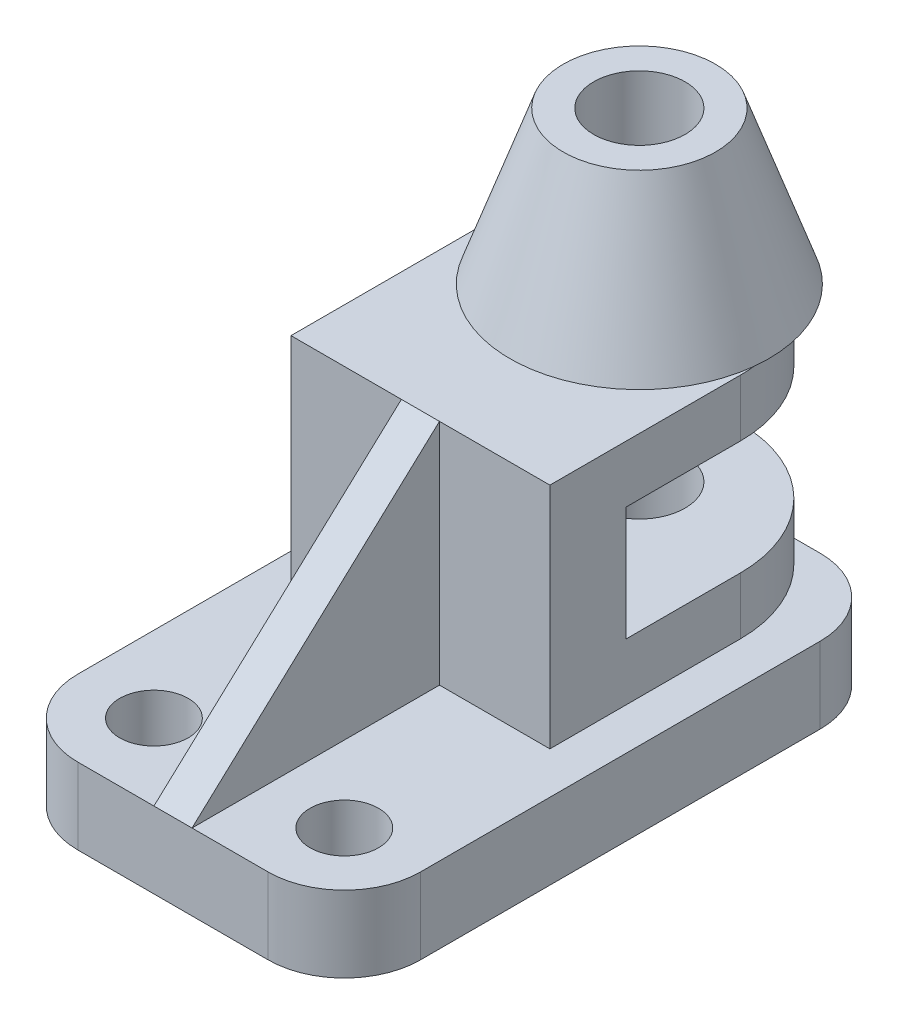
ISO-10303-21;
HEADER;
FILE_DESCRIPTION(('STEP AP214'),'2;1');
FILE_NAME('part.step','',(''),(''),'','','');
FILE_SCHEMA(('AUTOMOTIVE_DESIGN { 1 0 10303 214 1 1 1 1 }'));
ENDSEC;
DATA;
#1=APPLICATION_CONTEXT('core data for automotive mechanical design processes');
#2=APPLICATION_PROTOCOL_DEFINITION('international standard','automotive_design',2000,#1);
#3=PRODUCT_CONTEXT('',#1,'mechanical');
#4=PRODUCT('Part','Part','',(#3));
#5=PRODUCT_RELATED_PRODUCT_CATEGORY('part','',(#4));
#6=PRODUCT_DEFINITION_FORMATION('','',#4);
#7=PRODUCT_DEFINITION_CONTEXT('part definition',#1,'design');
#8=PRODUCT_DEFINITION('design','',#6,#7);
#9=PRODUCT_DEFINITION_SHAPE('','',#8);
#10=(LENGTH_UNIT() NAMED_UNIT(*) SI_UNIT(.MILLI.,.METRE.));
#11=(NAMED_UNIT(*) PLANE_ANGLE_UNIT() SI_UNIT($,.RADIAN.));
#12=(NAMED_UNIT(*) SI_UNIT($,.STERADIAN.) SOLID_ANGLE_UNIT());
#13=UNCERTAINTY_MEASURE_WITH_UNIT(LENGTH_MEASURE(1.E-05),#10,'distance_accuracy_value','');
#14=(GEOMETRIC_REPRESENTATION_CONTEXT(3) GLOBAL_UNCERTAINTY_ASSIGNED_CONTEXT((#13)) GLOBAL_UNIT_ASSIGNED_CONTEXT((#10,
#11,#12)) REPRESENTATION_CONTEXT('',''));
#15=CARTESIAN_POINT('',(0.,0.,0.));
#16=DIRECTION('',(0.,0.,1.));
#17=DIRECTION('',(1.,0.,0.));
#18=AXIS2_PLACEMENT_3D('',#15,#16,#17);
#19=CARTESIAN_POINT('',(0.,20.,0.));
#20=DIRECTION('',(0.,-1.,0.));
#21=DIRECTION('',(0.,0.,-1.));
#22=AXIS2_PLACEMENT_3D('',#19,#20,#21);
#23=PLANE('',#22);
#24=CARTESIAN_POINT('',(-25.,20.,52.5));
#25=DIRECTION('',(0.,1.,0.));
#26=DIRECTION('',(0.,0.,1.));
#27=AXIS2_PLACEMENT_3D('',#24,#25,#26);
#28=CIRCLE('',#27,9.);
#29=CARTESIAN_POINT('',(-25.,20.,61.5));
#30=VERTEX_POINT('',#29);
#31=EDGE_CURVE('E240',#30,#30,#28,.T.);
#32=ORIENTED_EDGE('',*,*,#31,.F.);
#33=EDGE_LOOP('',(#32));
#34=FACE_BOUND('',#33,.T.);
#35=DIRECTION('',(0.,0.,1.));
#36=VECTOR('',#35,1.);
#37=CARTESIAN_POINT('',(-5.,20.,0.));
#38=LINE('',#37,#36);
#39=CARTESIAN_POINT('',(-5.,20.,7.50000000000001));
#40=VERTEX_POINT('',#39);
#41=CARTESIAN_POINT('',(-5.,20.,72.5));
#42=VERTEX_POINT('',#41);
#43=EDGE_CURVE('E186',#40,#42,#38,.T.);
#44=ORIENTED_EDGE('',*,*,#43,.F.);
#45=DIRECTION('',(1.,0.,0.));
#46=VECTOR('',#45,1.);
#47=CARTESIAN_POINT('',(-34.,20.,7.50000000000001));
#48=LINE('',#47,#46);
#49=CARTESIAN_POINT('',(-34.,20.,7.50000000000001));
#50=VERTEX_POINT('',#49);
#51=EDGE_CURVE('E507',#50,#40,#48,.T.);
#52=ORIENTED_EDGE('',*,*,#51,.F.);
#53=DIRECTION('',(0.,0.,1.));
#54=VECTOR('',#53,1.);
#55=CARTESIAN_POINT('',(-34.,20.,-42.5));
#56=LINE('',#55,#54);
#57=CARTESIAN_POINT('',(-34.,20.,-42.5));
#58=VERTEX_POINT('',#57);
#59=EDGE_CURVE('E492',#58,#50,#56,.T.);
#60=ORIENTED_EDGE('',*,*,#59,.F.);
#61=CARTESIAN_POINT('',(0.,20.,-42.5));
#62=DIRECTION('',(0.,1.,0.));
#63=DIRECTION('',(0.,0.,1.));
#64=AXIS2_PLACEMENT_3D('',#61,#62,#63);
#65=CIRCLE('',#64,34.);
#66=CARTESIAN_POINT('',(-16.,20.,-72.5));
#67=VERTEX_POINT('',#66);
#68=EDGE_CURVE('E11',#67,#58,#65,.T.);
#69=ORIENTED_EDGE('',*,*,#68,.F.);
#70=DIRECTION('',(-1.,0.,0.));
#71=VECTOR('',#70,1.);
#72=CARTESIAN_POINT('',(-45.,20.,-72.5));
#73=LINE('',#72,#71);
#74=CARTESIAN_POINT('',(-25.,20.,-72.5));
#75=VERTEX_POINT('',#74);
#76=EDGE_CURVE('E225',#67,#75,#73,.T.);
#77=ORIENTED_EDGE('',*,*,#76,.T.);
#78=CARTESIAN_POINT('',(-25.,20.,-52.5));
#79=DIRECTION('',(0.,-1.,0.));
#80=DIRECTION('',(0.,0.,-1.));
#81=AXIS2_PLACEMENT_3D('',#78,#79,#80);
#82=CIRCLE('',#81,20.);
#83=CARTESIAN_POINT('',(-45.,20.,-52.5));
#84=VERTEX_POINT('',#83);
#85=EDGE_CURVE('E267',#75,#84,#82,.F.);
#86=ORIENTED_EDGE('',*,*,#85,.T.);
#87=DIRECTION('',(0.,0.,1.));
#88=VECTOR('',#87,1.);
#89=CARTESIAN_POINT('',(-45.,20.,72.5));
#90=LINE('',#89,#88);
#91=CARTESIAN_POINT('',(-45.,20.,52.5));
#92=VERTEX_POINT('',#91);
#93=EDGE_CURVE('E221',#84,#92,#90,.T.);
#94=ORIENTED_EDGE('',*,*,#93,.T.);
#95=CARTESIAN_POINT('',(-25.,20.,52.5));
#96=DIRECTION('',(0.,-1.,0.));
#97=DIRECTION('',(0.,0.,-1.));
#98=AXIS2_PLACEMENT_3D('',#95,#96,#97);
#99=CIRCLE('',#98,20.);
#100=CARTESIAN_POINT('',(-25.,20.,72.5));
#101=VERTEX_POINT('',#100);
#102=EDGE_CURVE('E217',#92,#101,#99,.F.);
#103=ORIENTED_EDGE('',*,*,#102,.T.);
#104=DIRECTION('',(1.,0.,0.));
#105=VECTOR('',#104,1.);
#106=CARTESIAN_POINT('',(-45.,20.,72.5));
#107=LINE('',#106,#105);
#108=EDGE_CURVE('E209',#101,#42,#107,.T.);
#109=ORIENTED_EDGE('',*,*,#108,.T.);
#110=EDGE_LOOP('',(#44,#52,#60,#69,#77,#86,#94,#103,#109));
#111=FACE_BOUND('',#110,.T.);
#112=ADVANCED_FACE('F43',(#34,#111),#23,.F.);
#113=CARTESIAN_POINT('',(-34.,80.,7.50000000000001));
#114=DIRECTION('',(0.,0.,-1.));
#115=DIRECTION('',(-1.,0.,0.));
#116=AXIS2_PLACEMENT_3D('',#113,#114,#115);
#117=PLANE('',#116);
#118=DIRECTION('',(0.,-1.,0.));
#119=VECTOR('',#118,1.);
#120=CARTESIAN_POINT('',(-5.,80.,7.50000000000001));
#121=LINE('',#120,#119);
#122=CARTESIAN_POINT('',(-5.,80.,7.49999999999999));
#123=VERTEX_POINT('',#122);
#124=EDGE_CURVE('E191',#123,#40,#121,.T.);
#125=ORIENTED_EDGE('',*,*,#124,.F.);
#126=DIRECTION('',(1.,0.,0.));
#127=VECTOR('',#126,1.);
#128=CARTESIAN_POINT('',(-34.,80.,7.50000000000001));
#129=LINE('',#128,#127);
#130=CARTESIAN_POINT('',(-34.,80.,7.50000000000001));
#131=VERTEX_POINT('',#130);
#132=EDGE_CURVE('E443',#131,#123,#129,.T.);
#133=ORIENTED_EDGE('',*,*,#132,.F.);
#134=DIRECTION('',(0.,-1.,0.));
#135=VECTOR('',#134,1.);
#136=CARTESIAN_POINT('',(-34.,80.,7.50000000000001));
#137=LINE('',#136,#135);
#138=EDGE_CURVE('E362',#131,#50,#137,.T.);
#139=ORIENTED_EDGE('',*,*,#138,.T.);
#140=ORIENTED_EDGE('',*,*,#51,.T.);
#141=EDGE_LOOP('',(#125,#133,#139,#140));
#142=FACE_BOUND('',#141,.T.);
#143=ADVANCED_FACE('F327',(#142),#117,.F.);
#144=CARTESIAN_POINT('',(-34.,80.,-42.5));
#145=DIRECTION('',(1.,0.,0.));
#146=DIRECTION('',(0.,0.,-1.));
#147=AXIS2_PLACEMENT_3D('',#144,#145,#146);
#148=PLANE('',#147);
#149=DIRECTION('',(0.,0.,1.));
#150=VECTOR('',#149,1.);
#151=CARTESIAN_POINT('',(-34.,35.,0.));
#152=LINE('',#151,#150);
#153=CARTESIAN_POINT('',(-34.,35.,-42.5));
#154=VERTEX_POINT('',#153);
#155=CARTESIAN_POINT('',(-34.,35.,-12.5));
#156=VERTEX_POINT('',#155);
#157=EDGE_CURVE('E473',#154,#156,#152,.T.);
#158=ORIENTED_EDGE('',*,*,#157,.F.);
#159=DIRECTION('',(0.,-1.,0.));
#160=VECTOR('',#159,1.);
#161=CARTESIAN_POINT('',(-34.,80.,-42.5));
#162=LINE('',#161,#160);
#163=EDGE_CURVE('E504',#154,#58,#162,.T.);
#164=ORIENTED_EDGE('',*,*,#163,.T.);
#165=ORIENTED_EDGE('',*,*,#59,.T.);
#166=ORIENTED_EDGE('',*,*,#138,.F.);
#167=DIRECTION('',(0.,0.,1.));
#168=VECTOR('',#167,1.);
#169=CARTESIAN_POINT('',(-34.,80.,-42.5));
#170=LINE('',#169,#168);
#171=CARTESIAN_POINT('',(-34.,80.,-42.5));
#172=VERTEX_POINT('',#171);
#173=EDGE_CURVE('E447',#172,#131,#170,.T.);
#174=ORIENTED_EDGE('',*,*,#173,.F.);
#175=CARTESIAN_POINT('',(-34.,65.,-42.5));
#176=VERTEX_POINT('',#175);
#177=EDGE_CURVE('E515',#172,#176,#162,.T.);
#178=ORIENTED_EDGE('',*,*,#177,.T.);
#179=DIRECTION('',(0.,0.,1.));
#180=VECTOR('',#179,1.);
#181=CARTESIAN_POINT('',(-34.,65.,0.));
#182=LINE('',#181,#180);
#183=CARTESIAN_POINT('',(-34.,65.,-12.5));
#184=VERTEX_POINT('',#183);
#185=EDGE_CURVE('E468',#176,#184,#182,.T.);
#186=ORIENTED_EDGE('',*,*,#185,.T.);
#187=DIRECTION('',(0.,1.,0.));
#188=VECTOR('',#187,1.);
#189=CARTESIAN_POINT('',(-34.,35.,-12.5));
#190=LINE('',#189,#188);
#191=EDGE_CURVE('E481',#156,#184,#190,.T.);
#192=ORIENTED_EDGE('',*,*,#191,.F.);
#193=EDGE_LOOP('',(#158,#164,#165,#166,#174,#178,#186,#192));
#194=FACE_BOUND('',#193,.T.);
#195=ADVANCED_FACE('F331',(#194),#148,.F.);
#196=CARTESIAN_POINT('',(34.,80.,7.50000000000001));
#197=DIRECTION('',(-1.,0.,0.));
#198=DIRECTION('',(0.,0.,1.));
#199=AXIS2_PLACEMENT_3D('',#196,#197,#198);
#200=PLANE('',#199);
#201=DIRECTION('',(0.,0.,-1.));
#202=VECTOR('',#201,1.);
#203=CARTESIAN_POINT('',(34.,35.,0.));
#204=LINE('',#203,#202);
#205=CARTESIAN_POINT('',(34.,35.,-12.5));
#206=VERTEX_POINT('',#205);
#207=CARTESIAN_POINT('',(34.,35.,-42.5));
#208=VERTEX_POINT('',#207);
#209=EDGE_CURVE('E480',#206,#208,#204,.T.);
#210=ORIENTED_EDGE('',*,*,#209,.F.);
#211=DIRECTION('',(0.,1.,0.));
#212=VECTOR('',#211,1.);
#213=CARTESIAN_POINT('',(34.,35.,-12.5));
#214=LINE('',#213,#212);
#215=CARTESIAN_POINT('',(34.,65.,-12.5));
#216=VERTEX_POINT('',#215);
#217=EDGE_CURVE('E489',#206,#216,#214,.T.);
#218=ORIENTED_EDGE('',*,*,#217,.T.);
#219=DIRECTION('',(0.,0.,-1.));
#220=VECTOR('',#219,1.);
#221=CARTESIAN_POINT('',(34.,65.,0.));
#222=LINE('',#221,#220);
#223=CARTESIAN_POINT('',(34.,65.,-42.5));
#224=VERTEX_POINT('',#223);
#225=EDGE_CURVE('E486',#216,#224,#222,.T.);
#226=ORIENTED_EDGE('',*,*,#225,.T.);
#227=DIRECTION('',(0.,-1.,0.));
#228=VECTOR('',#227,1.);
#229=CARTESIAN_POINT('',(34.,80.,-42.5));
#230=LINE('',#229,#228);
#231=CARTESIAN_POINT('',(34.,80.,-42.5));
#232=VERTEX_POINT('',#231);
#233=EDGE_CURVE('E517',#232,#224,#230,.T.);
#234=ORIENTED_EDGE('',*,*,#233,.F.);
#235=DIRECTION('',(0.,0.,-1.));
#236=VECTOR('',#235,1.);
#237=CARTESIAN_POINT('',(34.,80.,7.50000000000001));
#238=LINE('',#237,#236);
#239=CARTESIAN_POINT('',(34.,80.,7.50000000000001));
#240=VERTEX_POINT('',#239);
#241=EDGE_CURVE('E497',#240,#232,#238,.T.);
#242=ORIENTED_EDGE('',*,*,#241,.F.);
#243=DIRECTION('',(0.,-1.,0.));
#244=VECTOR('',#243,1.);
#245=CARTESIAN_POINT('',(34.,80.,7.50000000000001));
#246=LINE('',#245,#244);
#247=CARTESIAN_POINT('',(34.,20.,7.50000000000001));
#248=VERTEX_POINT('',#247);
#249=EDGE_CURVE('E444',#240,#248,#246,.T.);
#250=ORIENTED_EDGE('',*,*,#249,.T.);
#251=DIRECTION('',(0.,0.,-1.));
#252=VECTOR('',#251,1.);
#253=CARTESIAN_POINT('',(34.,20.,7.50000000000001));
#254=LINE('',#253,#252);
#255=CARTESIAN_POINT('',(34.,20.,-42.5));
#256=VERTEX_POINT('',#255);
#257=EDGE_CURVE('E510',#248,#256,#254,.T.);
#258=ORIENTED_EDGE('',*,*,#257,.T.);
#259=EDGE_CURVE('E513',#208,#256,#230,.T.);
#260=ORIENTED_EDGE('',*,*,#259,.F.);
#261=EDGE_LOOP('',(#210,#218,#226,#234,#242,#250,#258,#260));
#262=FACE_BOUND('',#261,.T.);
#263=ADVANCED_FACE('F349',(#262),#200,.F.);
#264=CARTESIAN_POINT('',(0.,80.,-42.5));
#265=DIRECTION('',(0.,-1.,0.));
#266=DIRECTION('',(0.,0.,-1.));
#267=AXIS2_PLACEMENT_3D('',#264,#265,#266);
#268=CYLINDRICAL_SURFACE('',#267,34.);
#269=CARTESIAN_POINT('',(16.,20.,-72.5));
#270=VERTEX_POINT('',#269);
#271=EDGE_CURVE('E53',#270,#67,#65,.T.);
#272=ORIENTED_EDGE('',*,*,#271,.T.);
#273=ORIENTED_EDGE('',*,*,#68,.T.);
#274=ORIENTED_EDGE('',*,*,#163,.F.);
#275=CARTESIAN_POINT('',(0.,35.,-42.5));
#276=DIRECTION('',(0.,1.,0.));
#277=DIRECTION('',(0.,0.,1.));
#278=AXIS2_PLACEMENT_3D('',#275,#276,#277);
#279=CIRCLE('',#278,34.);
#280=EDGE_CURVE('E479',#208,#154,#279,.T.);
#281=ORIENTED_EDGE('',*,*,#280,.F.);
#282=ORIENTED_EDGE('',*,*,#259,.T.);
#283=EDGE_CURVE('E52',#256,#270,#65,.T.);
#284=ORIENTED_EDGE('',*,*,#283,.T.);
#285=EDGE_LOOP('',(#272,#273,#274,#281,#282,#284));
#286=FACE_BOUND('',#285,.T.);
#287=ADVANCED_FACE('F344',(#286),#268,.T.);
#288=CARTESIAN_POINT('',(25.,20.,52.5));
#289=DIRECTION('',(0.,1.,0.));
#290=DIRECTION('',(0.,0.,1.));
#291=AXIS2_PLACEMENT_3D('',#288,#289,#290);
#292=CIRCLE('',#291,9.);
#293=CARTESIAN_POINT('',(25.,20.,61.5));
#294=VERTEX_POINT('',#293);
#295=EDGE_CURVE('E353',#294,#294,#292,.T.);
#296=ORIENTED_EDGE('',*,*,#295,.F.);
#297=EDGE_LOOP('',(#296));
#298=FACE_BOUND('',#297,.T.);
#299=CARTESIAN_POINT('',(5.,20.,7.50000000000001));
#300=VERTEX_POINT('',#299);
#301=EDGE_CURVE('E503',#300,#248,#48,.T.);
#302=ORIENTED_EDGE('',*,*,#301,.F.);
#303=DIRECTION('',(0.,0.,1.));
#304=VECTOR('',#303,1.);
#305=CARTESIAN_POINT('',(5.,20.,0.));
#306=LINE('',#305,#304);
#307=CARTESIAN_POINT('',(5.,20.,72.5));
#308=VERTEX_POINT('',#307);
#309=EDGE_CURVE('E437',#300,#308,#306,.T.);
#310=ORIENTED_EDGE('',*,*,#309,.T.);
#311=CARTESIAN_POINT('',(25.,20.,72.5));
#312=VERTEX_POINT('',#311);
#313=EDGE_CURVE('E213',#308,#312,#107,.T.);
#314=ORIENTED_EDGE('',*,*,#313,.T.);
#315=CARTESIAN_POINT('',(25.,20.,52.5));
#316=DIRECTION('',(0.,-1.,0.));
#317=DIRECTION('',(0.,0.,-1.));
#318=AXIS2_PLACEMENT_3D('',#315,#316,#317);
#319=CIRCLE('',#318,20.);
#320=CARTESIAN_POINT('',(45.,20.,52.5));
#321=VERTEX_POINT('',#320);
#322=EDGE_CURVE('E262',#312,#321,#319,.F.);
#323=ORIENTED_EDGE('',*,*,#322,.T.);
#324=DIRECTION('',(0.,0.,-1.));
#325=VECTOR('',#324,1.);
#326=CARTESIAN_POINT('',(45.,20.,72.5));
#327=LINE('',#326,#325);
#328=CARTESIAN_POINT('',(45.,20.,-52.5));
#329=VERTEX_POINT('',#328);
#330=EDGE_CURVE('E218',#321,#329,#327,.T.);
#331=ORIENTED_EDGE('',*,*,#330,.T.);
#332=CARTESIAN_POINT('',(25.,20.,-52.5));
#333=DIRECTION('',(0.,-1.,0.));
#334=DIRECTION('',(0.,0.,-1.));
#335=AXIS2_PLACEMENT_3D('',#332,#333,#334);
#336=CIRCLE('',#335,20.);
#337=CARTESIAN_POINT('',(24.9999999999999,20.,-72.5));
#338=VERTEX_POINT('',#337);
#339=EDGE_CURVE('E270',#329,#338,#336,.F.);
#340=ORIENTED_EDGE('',*,*,#339,.T.);
#341=EDGE_CURVE('E230',#338,#270,#73,.T.);
#342=ORIENTED_EDGE('',*,*,#341,.T.);
#343=ORIENTED_EDGE('',*,*,#283,.F.);
#344=ORIENTED_EDGE('',*,*,#257,.F.);
#345=EDGE_LOOP('',(#302,#310,#314,#323,#331,#340,#342,#343,#344));
#346=FACE_BOUND('',#345,.T.);
#347=ADVANCED_FACE('F288',(#298,#346),#23,.F.);
#348=CARTESIAN_POINT('',(0.,0.,0.));
#349=DIRECTION('',(0.,-1.,0.));
#350=DIRECTION('',(0.,0.,-1.));
#351=AXIS2_PLACEMENT_3D('',#348,#349,#350);
#352=PLANE('',#351);
#353=CARTESIAN_POINT('',(0.,0.,-50.));
#354=DIRECTION('',(0.,1.,0.));
#355=DIRECTION('',(0.,0.,1.));
#356=AXIS2_PLACEMENT_3D('',#353,#354,#355);
#357=CIRCLE('',#356,12.);
#358=CARTESIAN_POINT('',(0.,0.,-38.));
#359=VERTEX_POINT('',#358);
#360=EDGE_CURVE('E455',#359,#359,#357,.T.);
#361=ORIENTED_EDGE('',*,*,#360,.T.);
#362=EDGE_LOOP('',(#361));
#363=FACE_BOUND('',#362,.T.);
#364=CARTESIAN_POINT('',(-25.,0.,-52.5));
#365=DIRECTION('',(0.,-1.,0.));
#366=DIRECTION('',(0.,0.,-1.));
#367=AXIS2_PLACEMENT_3D('',#364,#365,#366);
#368=CIRCLE('',#367,20.);
#369=CARTESIAN_POINT('',(-45.,0.,-52.5));
#370=VERTEX_POINT('',#369);
#371=CARTESIAN_POINT('',(-25.,0.,-72.5));
#372=VERTEX_POINT('',#371);
#373=EDGE_CURVE('E254',#370,#372,#368,.T.);
#374=ORIENTED_EDGE('',*,*,#373,.T.);
#375=DIRECTION('',(-1.,0.,0.));
#376=VECTOR('',#375,1.);
#377=CARTESIAN_POINT('',(-45.,0.,-72.5));
#378=LINE('',#377,#376);
#379=CARTESIAN_POINT('',(24.9999999999999,0.,-72.5));
#380=VERTEX_POINT('',#379);
#381=EDGE_CURVE('E244',#380,#372,#378,.T.);
#382=ORIENTED_EDGE('',*,*,#381,.F.);
#383=CARTESIAN_POINT('',(25.,0.,-52.5));
#384=DIRECTION('',(0.,-1.,0.));
#385=DIRECTION('',(0.,0.,-1.));
#386=AXIS2_PLACEMENT_3D('',#383,#384,#385);
#387=CIRCLE('',#386,20.);
#388=CARTESIAN_POINT('',(45.,0.,-52.5));
#389=VERTEX_POINT('',#388);
#390=EDGE_CURVE('E251',#380,#389,#387,.T.);
#391=ORIENTED_EDGE('',*,*,#390,.T.);
#392=DIRECTION('',(0.,0.,-1.));
#393=VECTOR('',#392,1.);
#394=CARTESIAN_POINT('',(45.,0.,72.5));
#395=LINE('',#394,#393);
#396=CARTESIAN_POINT('',(45.,0.,52.5));
#397=VERTEX_POINT('',#396);
#398=EDGE_CURVE('E239',#397,#389,#395,.T.);
#399=ORIENTED_EDGE('',*,*,#398,.F.);
#400=CARTESIAN_POINT('',(25.,0.,52.5));
#401=DIRECTION('',(0.,-1.,0.));
#402=DIRECTION('',(0.,0.,-1.));
#403=AXIS2_PLACEMENT_3D('',#400,#401,#402);
#404=CIRCLE('',#403,20.);
#405=CARTESIAN_POINT('',(25.,0.,72.5));
#406=VERTEX_POINT('',#405);
#407=EDGE_CURVE('E250',#397,#406,#404,.T.);
#408=ORIENTED_EDGE('',*,*,#407,.T.);
#409=DIRECTION('',(1.,0.,0.));
#410=VECTOR('',#409,1.);
#411=CARTESIAN_POINT('',(-45.,0.,72.5));
#412=LINE('',#411,#410);
#413=CARTESIAN_POINT('',(-25.,0.,72.5));
#414=VERTEX_POINT('',#413);
#415=EDGE_CURVE('E237',#414,#406,#412,.T.);
#416=ORIENTED_EDGE('',*,*,#415,.F.);
#417=CARTESIAN_POINT('',(-25.,0.,52.5));
#418=DIRECTION('',(0.,-1.,0.));
#419=DIRECTION('',(0.,0.,-1.));
#420=AXIS2_PLACEMENT_3D('',#417,#418,#419);
#421=CIRCLE('',#420,20.);
#422=CARTESIAN_POINT('',(-45.,0.,52.5));
#423=VERTEX_POINT('',#422);
#424=EDGE_CURVE('E253',#414,#423,#421,.T.);
#425=ORIENTED_EDGE('',*,*,#424,.T.);
#426=DIRECTION('',(0.,0.,1.));
#427=VECTOR('',#426,1.);
#428=CARTESIAN_POINT('',(-45.,0.,72.5));
#429=LINE('',#428,#427);
#430=EDGE_CURVE('E235',#370,#423,#429,.T.);
#431=ORIENTED_EDGE('',*,*,#430,.F.);
#432=EDGE_LOOP('',(#374,#382,#391,#399,#408,#416,#425,#431));
#433=FACE_BOUND('',#432,.T.);
#434=CARTESIAN_POINT('',(25.,0.,52.5));
#435=DIRECTION('',(0.,1.,0.));
#436=DIRECTION('',(0.,0.,1.));
#437=AXIS2_PLACEMENT_3D('',#434,#435,#436);
#438=CIRCLE('',#437,9.);
#439=CARTESIAN_POINT('',(25.,0.,61.5));
#440=VERTEX_POINT('',#439);
#441=EDGE_CURVE('E360',#440,#440,#438,.T.);
#442=ORIENTED_EDGE('',*,*,#441,.T.);
#443=EDGE_LOOP('',(#442));
#444=FACE_BOUND('',#443,.T.);
#445=CARTESIAN_POINT('',(-25.,0.,52.5));
#446=DIRECTION('',(0.,1.,0.));
#447=DIRECTION('',(0.,0.,1.));
#448=AXIS2_PLACEMENT_3D('',#445,#446,#447);
#449=CIRCLE('',#448,9.);
#450=CARTESIAN_POINT('',(-25.,0.,61.5));
#451=VERTEX_POINT('',#450);
#452=EDGE_CURVE('E359',#451,#451,#449,.T.);
#453=ORIENTED_EDGE('',*,*,#452,.T.);
#454=EDGE_LOOP('',(#453));
#455=FACE_BOUND('',#454,.T.);
#456=ADVANCED_FACE('F282',(#363,#433,#444,#455),#352,.T.);
#457=CARTESIAN_POINT('',(-45.,20.,72.5));
#458=DIRECTION('',(1.,0.,0.));
#459=DIRECTION('',(0.,0.,-1.));
#460=AXIS2_PLACEMENT_3D('',#457,#458,#459);
#461=PLANE('',#460);
#462=ORIENTED_EDGE('',*,*,#93,.F.);
#463=DIRECTION('',(0.,-1.,0.));
#464=VECTOR('',#463,1.);
#465=CARTESIAN_POINT('',(-45.,20.,-52.5));
#466=LINE('',#465,#464);
#467=EDGE_CURVE('E243',#84,#370,#466,.T.);
#468=ORIENTED_EDGE('',*,*,#467,.T.);
#469=ORIENTED_EDGE('',*,*,#430,.T.);
#470=DIRECTION('',(0.,-1.,0.));
#471=VECTOR('',#470,1.);
#472=CARTESIAN_POINT('',(-45.,20.,52.5));
#473=LINE('',#472,#471);
#474=EDGE_CURVE('E232',#423,#92,#473,.F.);
#475=ORIENTED_EDGE('',*,*,#474,.T.);
#476=EDGE_LOOP('',(#462,#468,#469,#475));
#477=FACE_BOUND('',#476,.T.);
#478=ADVANCED_FACE('F320',(#477),#461,.F.);
#479=CARTESIAN_POINT('',(-45.,20.,72.5));
#480=DIRECTION('',(0.,0.,-1.));
#481=DIRECTION('',(-1.,0.,0.));
#482=AXIS2_PLACEMENT_3D('',#479,#480,#481);
#483=PLANE('',#482);
#484=ORIENTED_EDGE('',*,*,#313,.F.);
#485=DIRECTION('',(-1.,0.,0.));
#486=VECTOR('',#485,1.);
#487=CARTESIAN_POINT('',(-45.,20.,72.5));
#488=LINE('',#487,#486);
#489=EDGE_CURVE('E203',#42,#308,#488,.F.);
#490=ORIENTED_EDGE('',*,*,#489,.F.);
#491=ORIENTED_EDGE('',*,*,#108,.F.);
#492=DIRECTION('',(0.,-1.,0.));
#493=VECTOR('',#492,1.);
#494=CARTESIAN_POINT('',(-25.,20.,72.5));
#495=LINE('',#494,#493);
#496=EDGE_CURVE('E50',#101,#414,#495,.T.);
#497=ORIENTED_EDGE('',*,*,#496,.T.);
#498=ORIENTED_EDGE('',*,*,#415,.T.);
#499=DIRECTION('',(0.,-1.,0.));
#500=VECTOR('',#499,1.);
#501=CARTESIAN_POINT('',(25.,20.,72.5));
#502=LINE('',#501,#500);
#503=EDGE_CURVE('E274',#406,#312,#502,.F.);
#504=ORIENTED_EDGE('',*,*,#503,.T.);
#505=EDGE_LOOP('',(#484,#490,#491,#497,#498,#504));
#506=FACE_BOUND('',#505,.T.);
#507=ADVANCED_FACE('F208',(#506),#483,.F.);
#508=CARTESIAN_POINT('',(45.,20.,72.5));
#509=DIRECTION('',(-1.,0.,0.));
#510=DIRECTION('',(0.,0.,1.));
#511=AXIS2_PLACEMENT_3D('',#508,#509,#510);
#512=PLANE('',#511);
#513=ORIENTED_EDGE('',*,*,#398,.T.);
#514=DIRECTION('',(0.,-1.,0.));
#515=VECTOR('',#514,1.);
#516=CARTESIAN_POINT('',(45.,20.,-52.5));
#517=LINE('',#516,#515);
#518=EDGE_CURVE('E273',#389,#329,#517,.F.);
#519=ORIENTED_EDGE('',*,*,#518,.T.);
#520=ORIENTED_EDGE('',*,*,#330,.F.);
#521=DIRECTION('',(0.,-1.,0.));
#522=VECTOR('',#521,1.);
#523=CARTESIAN_POINT('',(45.,20.,52.5));
#524=LINE('',#523,#522);
#525=EDGE_CURVE('E271',#321,#397,#524,.T.);
#526=ORIENTED_EDGE('',*,*,#525,.T.);
#527=EDGE_LOOP('',(#513,#519,#520,#526));
#528=FACE_BOUND('',#527,.T.);
#529=ADVANCED_FACE('F294',(#528),#512,.F.);
#530=CARTESIAN_POINT('',(-45.,20.,-72.5));
#531=DIRECTION('',(0.,0.,1.));
#532=DIRECTION('',(1.,0.,0.));
#533=AXIS2_PLACEMENT_3D('',#530,#531,#532);
#534=PLANE('',#533);
#535=ORIENTED_EDGE('',*,*,#381,.T.);
#536=DIRECTION('',(0.,-1.,0.));
#537=VECTOR('',#536,1.);
#538=CARTESIAN_POINT('',(-25.,20.,-72.5));
#539=LINE('',#538,#537);
#540=EDGE_CURVE('E261',#372,#75,#539,.F.);
#541=ORIENTED_EDGE('',*,*,#540,.T.);
#542=ORIENTED_EDGE('',*,*,#76,.F.);
#543=EDGE_CURVE('E234',#270,#67,#73,.T.);
#544=ORIENTED_EDGE('',*,*,#543,.F.);
#545=ORIENTED_EDGE('',*,*,#341,.F.);
#546=DIRECTION('',(0.,-1.,0.));
#547=VECTOR('',#546,1.);
#548=CARTESIAN_POINT('',(25.,20.,-72.5));
#549=LINE('',#548,#547);
#550=EDGE_CURVE('E256',#338,#380,#549,.T.);
#551=ORIENTED_EDGE('',*,*,#550,.T.);
#552=EDGE_LOOP('',(#535,#541,#542,#544,#545,#551));
#553=FACE_BOUND('',#552,.T.);
#554=ADVANCED_FACE('F305',(#553),#534,.F.);
#555=CARTESIAN_POINT('',(-25.,20.,52.5));
#556=DIRECTION('',(0.,-1.,0.));
#557=DIRECTION('',(0.,0.,-1.));
#558=AXIS2_PLACEMENT_3D('',#555,#556,#557);
#559=CYLINDRICAL_SURFACE('',#558,9.);
#560=ORIENTED_EDGE('',*,*,#31,.T.);
#561=EDGE_LOOP('',(#560));
#562=FACE_BOUND('',#561,.T.);
#563=ORIENTED_EDGE('',*,*,#452,.F.);
#564=EDGE_LOOP('',(#563));
#565=FACE_BOUND('',#564,.T.);
#566=ADVANCED_FACE('F369',(#562,#565),#559,.F.);
#567=CARTESIAN_POINT('',(25.,20.,52.5));
#568=DIRECTION('',(0.,-1.,0.));
#569=DIRECTION('',(0.,0.,-1.));
#570=AXIS2_PLACEMENT_3D('',#567,#568,#569);
#571=CYLINDRICAL_SURFACE('',#570,9.);
#572=ORIENTED_EDGE('',*,*,#295,.T.);
#573=EDGE_LOOP('',(#572));
#574=FACE_BOUND('',#573,.T.);
#575=ORIENTED_EDGE('',*,*,#441,.F.);
#576=EDGE_LOOP('',(#575));
#577=FACE_BOUND('',#576,.T.);
#578=ADVANCED_FACE('F375',(#574,#577),#571,.F.);
#579=CARTESIAN_POINT('',(-25.,20.,-52.5));
#580=DIRECTION('',(0.,-1.,0.));
#581=DIRECTION('',(0.,0.,-1.));
#582=AXIS2_PLACEMENT_3D('',#579,#580,#581);
#583=CYLINDRICAL_SURFACE('',#582,20.);
#584=ORIENTED_EDGE('',*,*,#85,.F.);
#585=ORIENTED_EDGE('',*,*,#540,.F.);
#586=ORIENTED_EDGE('',*,*,#373,.F.);
#587=ORIENTED_EDGE('',*,*,#467,.F.);
#588=EDGE_LOOP('',(#584,#585,#586,#587));
#589=FACE_BOUND('',#588,.T.);
#590=ADVANCED_FACE('F312',(#589),#583,.T.);
#591=CARTESIAN_POINT('',(25.,20.,-52.5));
#592=DIRECTION('',(0.,-1.,0.));
#593=DIRECTION('',(0.,0.,-1.));
#594=AXIS2_PLACEMENT_3D('',#591,#592,#593);
#595=CYLINDRICAL_SURFACE('',#594,20.);
#596=ORIENTED_EDGE('',*,*,#339,.F.);
#597=ORIENTED_EDGE('',*,*,#518,.F.);
#598=ORIENTED_EDGE('',*,*,#390,.F.);
#599=ORIENTED_EDGE('',*,*,#550,.F.);
#600=EDGE_LOOP('',(#596,#597,#598,#599));
#601=FACE_BOUND('',#600,.T.);
#602=ADVANCED_FACE('F299',(#601),#595,.T.);
#603=CARTESIAN_POINT('',(-25.,20.,52.5));
#604=DIRECTION('',(0.,-1.,0.));
#605=DIRECTION('',(0.,0.,-1.));
#606=AXIS2_PLACEMENT_3D('',#603,#604,#605);
#607=CYLINDRICAL_SURFACE('',#606,20.);
#608=ORIENTED_EDGE('',*,*,#102,.F.);
#609=ORIENTED_EDGE('',*,*,#474,.F.);
#610=ORIENTED_EDGE('',*,*,#424,.F.);
#611=ORIENTED_EDGE('',*,*,#496,.F.);
#612=EDGE_LOOP('',(#608,#609,#610,#611));
#613=FACE_BOUND('',#612,.T.);
#614=ADVANCED_FACE('F317',(#613),#607,.T.);
#615=CARTESIAN_POINT('',(25.,20.,52.5));
#616=DIRECTION('',(0.,-1.,0.));
#617=DIRECTION('',(0.,0.,-1.));
#618=AXIS2_PLACEMENT_3D('',#615,#616,#617);
#619=CYLINDRICAL_SURFACE('',#618,20.);
#620=ORIENTED_EDGE('',*,*,#322,.F.);
#621=ORIENTED_EDGE('',*,*,#503,.F.);
#622=ORIENTED_EDGE('',*,*,#407,.F.);
#623=ORIENTED_EDGE('',*,*,#525,.F.);
#624=EDGE_LOOP('',(#620,#621,#622,#623));
#625=FACE_BOUND('',#624,.T.);
#626=ADVANCED_FACE('F44',(#625),#619,.T.);
#627=CARTESIAN_POINT('',(0.,20.,-42.5));
#628=DIRECTION('',(0.,1.,0.));
#629=DIRECTION('',(0.,0.,1.));
#630=AXIS2_PLACEMENT_3D('',#627,#628,#629);
#631=PLANE('',#630);
#632=ORIENTED_EDGE('',*,*,#543,.T.);
#633=ORIENTED_EDGE('',*,*,#271,.F.);
#634=EDGE_LOOP('',(#632,#633));
#635=FACE_BOUND('',#634,.T.);
#636=ADVANCED_FACE('F324',(#635),#631,.F.);
#637=CARTESIAN_POINT('',(5.,80.,7.50000000000001));
#638=VERTEX_POINT('',#637);
#639=EDGE_CURVE('E442',#638,#240,#129,.T.);
#640=ORIENTED_EDGE('',*,*,#639,.F.);
#641=DIRECTION('',(0.,-1.,0.));
#642=VECTOR('',#641,1.);
#643=CARTESIAN_POINT('',(5.,80.,7.50000000000001));
#644=LINE('',#643,#642);
#645=EDGE_CURVE('E436',#638,#300,#644,.T.);
#646=ORIENTED_EDGE('',*,*,#645,.T.);
#647=ORIENTED_EDGE('',*,*,#301,.T.);
#648=ORIENTED_EDGE('',*,*,#249,.F.);
#649=EDGE_LOOP('',(#640,#646,#647,#648));
#650=FACE_BOUND('',#649,.T.);
#651=ADVANCED_FACE('F339',(#650),#117,.F.);
#652=CARTESIAN_POINT('',(0.,65.,-42.5));
#653=DIRECTION('',(0.,1.,0.));
#654=DIRECTION('',(0.,0.,1.));
#655=AXIS2_PLACEMENT_3D('',#652,#653,#654);
#656=CIRCLE('',#655,34.);
#657=EDGE_CURVE('E474',#224,#176,#656,.T.);
#658=ORIENTED_EDGE('',*,*,#657,.T.);
#659=ORIENTED_EDGE('',*,*,#177,.F.);
#660=CARTESIAN_POINT('',(0.,80.,-42.5));
#661=DIRECTION('',(0.,1.,0.));
#662=DIRECTION('',(0.,0.,1.));
#663=AXIS2_PLACEMENT_3D('',#660,#661,#662);
#664=CIRCLE('',#663,34.);
#665=CARTESIAN_POINT('',(-33.7925657504724,80.,-46.2500000000001));
#666=VERTEX_POINT('',#665);
#667=EDGE_CURVE('E499',#666,#172,#664,.T.);
#668=ORIENTED_EDGE('',*,*,#667,.F.);
#669=CARTESIAN_POINT('',(33.7925657504724,80.,-46.25));
#670=VERTEX_POINT('',#669);
#671=EDGE_CURVE('E70',#670,#666,#664,.T.);
#672=ORIENTED_EDGE('',*,*,#671,.F.);
#673=EDGE_CURVE('E496',#232,#670,#664,.T.);
#674=ORIENTED_EDGE('',*,*,#673,.F.);
#675=ORIENTED_EDGE('',*,*,#233,.T.);
#676=EDGE_LOOP('',(#658,#659,#668,#672,#674,#675));
#677=FACE_BOUND('',#676,.T.);
#678=ADVANCED_FACE('F354',(#677),#268,.T.);
#679=CARTESIAN_POINT('',(0.,80.,-42.5));
#680=DIRECTION('',(0.,1.,0.));
#681=DIRECTION('',(0.,0.,1.));
#682=AXIS2_PLACEMENT_3D('',#679,#680,#681);
#683=PLANE('',#682);
#684=CARTESIAN_POINT('',(0.,80.,-50.));
#685=DIRECTION('',(0.,-1.,0.));
#686=DIRECTION('',(0.,0.,-1.));
#687=AXIS2_PLACEMENT_3D('',#684,#685,#686);
#688=CIRCLE('',#687,34.);
#689=EDGE_CURVE('E463',#670,#666,#688,.T.);
#690=ORIENTED_EDGE('',*,*,#689,.T.);
#691=ORIENTED_EDGE('',*,*,#667,.T.);
#692=ORIENTED_EDGE('',*,*,#173,.T.);
#693=ORIENTED_EDGE('',*,*,#132,.T.);
#694=DIRECTION('',(-1.,0.,0.));
#695=VECTOR('',#694,1.);
#696=CARTESIAN_POINT('',(0.,80.,7.50000000000001));
#697=LINE('',#696,#695);
#698=EDGE_CURVE('E201',#123,#638,#697,.F.);
#699=ORIENTED_EDGE('',*,*,#698,.T.);
#700=ORIENTED_EDGE('',*,*,#639,.T.);
#701=ORIENTED_EDGE('',*,*,#241,.T.);
#702=ORIENTED_EDGE('',*,*,#673,.T.);
#703=EDGE_LOOP('',(#690,#691,#692,#693,#699,#700,#701,#702));
#704=FACE_BOUND('',#703,.T.);
#705=ADVANCED_FACE('F392',(#704),#683,.T.);
#706=CARTESIAN_POINT('',(0.,35.,-12.5));
#707=DIRECTION('',(0.,0.,1.));
#708=DIRECTION('',(1.,0.,0.));
#709=AXIS2_PLACEMENT_3D('',#706,#707,#708);
#710=PLANE('',#709);
#711=ORIENTED_EDGE('',*,*,#217,.F.);
#712=DIRECTION('',(1.,0.,0.));
#713=VECTOR('',#712,1.);
#714=CARTESIAN_POINT('',(0.,35.,-12.5));
#715=LINE('',#714,#713);
#716=EDGE_CURVE('E475',#156,#206,#715,.T.);
#717=ORIENTED_EDGE('',*,*,#716,.F.);
#718=ORIENTED_EDGE('',*,*,#191,.T.);
#719=DIRECTION('',(1.,0.,0.));
#720=VECTOR('',#719,1.);
#721=CARTESIAN_POINT('',(0.,65.,-12.5));
#722=LINE('',#721,#720);
#723=EDGE_CURVE('E482',#184,#216,#722,.T.);
#724=ORIENTED_EDGE('',*,*,#723,.T.);
#725=EDGE_LOOP('',(#711,#717,#718,#724));
#726=FACE_BOUND('',#725,.T.);
#727=ADVANCED_FACE('F399',(#726),#710,.F.);
#728=CARTESIAN_POINT('',(0.,35.,0.));
#729=DIRECTION('',(0.,1.,0.));
#730=DIRECTION('',(0.,0.,1.));
#731=AXIS2_PLACEMENT_3D('',#728,#729,#730);
#732=PLANE('',#731);
#733=CARTESIAN_POINT('',(0.,35.,-50.));
#734=DIRECTION('',(0.,1.,0.));
#735=DIRECTION('',(0.,0.,1.));
#736=AXIS2_PLACEMENT_3D('',#733,#734,#735);
#737=CIRCLE('',#736,12.);
#738=CARTESIAN_POINT('',(0.,35.,-38.));
#739=VERTEX_POINT('',#738);
#740=EDGE_CURVE('E462',#739,#739,#737,.T.);
#741=ORIENTED_EDGE('',*,*,#740,.F.);
#742=EDGE_LOOP('',(#741));
#743=FACE_BOUND('',#742,.T.);
#744=ORIENTED_EDGE('',*,*,#716,.T.);
#745=ORIENTED_EDGE('',*,*,#209,.T.);
#746=ORIENTED_EDGE('',*,*,#280,.T.);
#747=ORIENTED_EDGE('',*,*,#157,.T.);
#748=EDGE_LOOP('',(#744,#745,#746,#747));
#749=FACE_BOUND('',#748,.T.);
#750=ADVANCED_FACE('F402',(#743,#749),#732,.T.);
#751=CARTESIAN_POINT('',(0.,65.,0.));
#752=DIRECTION('',(0.,1.,0.));
#753=DIRECTION('',(0.,0.,1.));
#754=AXIS2_PLACEMENT_3D('',#751,#752,#753);
#755=PLANE('',#754);
#756=CARTESIAN_POINT('',(0.,65.,-50.));
#757=DIRECTION('',(0.,1.,0.));
#758=DIRECTION('',(0.,0.,1.));
#759=AXIS2_PLACEMENT_3D('',#756,#757,#758);
#760=CIRCLE('',#759,12.);
#761=CARTESIAN_POINT('',(0.,65.,-38.));
#762=VERTEX_POINT('',#761);
#763=EDGE_CURVE('E457',#762,#762,#760,.T.);
#764=ORIENTED_EDGE('',*,*,#763,.T.);
#765=EDGE_LOOP('',(#764));
#766=FACE_BOUND('',#765,.T.);
#767=ORIENTED_EDGE('',*,*,#225,.F.);
#768=ORIENTED_EDGE('',*,*,#723,.F.);
#769=ORIENTED_EDGE('',*,*,#185,.F.);
#770=ORIENTED_EDGE('',*,*,#657,.F.);
#771=EDGE_LOOP('',(#767,#768,#769,#770));
#772=FACE_BOUND('',#771,.T.);
#773=ADVANCED_FACE('F401',(#766,#772),#755,.F.);
#774=CARTESIAN_POINT('',(34.,80.,-50.));
#775=DIRECTION('',(0.,-1.,0.));
#776=DIRECTION('',(0.,0.,-1.));
#777=AXIS2_PLACEMENT_3D('',#774,#775,#776);
#778=PLANE('',#777);
#779=ORIENTED_EDGE('',*,*,#671,.T.);
#780=EDGE_CURVE('E461',#666,#670,#688,.T.);
#781=ORIENTED_EDGE('',*,*,#780,.T.);
#782=EDGE_LOOP('',(#779,#781));
#783=FACE_BOUND('',#782,.T.);
#784=ADVANCED_FACE('F407',(#783),#778,.T.);
#785=CARTESIAN_POINT('',(0.,120.,-50.));
#786=DIRECTION('',(0.,1.,0.));
#787=DIRECTION('',(0.,0.,1.));
#788=AXIS2_PLACEMENT_3D('',#785,#786,#787);
#789=PLANE('',#788);
#790=CARTESIAN_POINT('',(0.,120.,-50.));
#791=DIRECTION('',(0.,1.,0.));
#792=DIRECTION('',(0.,0.,1.));
#793=AXIS2_PLACEMENT_3D('',#790,#791,#792);
#794=CIRCLE('',#793,12.);
#795=CARTESIAN_POINT('',(0.,120.,-38.));
#796=VERTEX_POINT('',#795);
#797=EDGE_CURVE('E212',#796,#796,#794,.T.);
#798=ORIENTED_EDGE('',*,*,#797,.F.);
#799=EDGE_LOOP('',(#798));
#800=FACE_BOUND('',#799,.T.);
#801=CARTESIAN_POINT('',(0.,120.,-50.));
#802=DIRECTION('',(0.,-1.,0.));
#803=DIRECTION('',(0.,0.,-1.));
#804=AXIS2_PLACEMENT_3D('',#801,#802,#803);
#805=CIRCLE('',#804,20.);
#806=CARTESIAN_POINT('',(0.,120.,-70.));
#807=VERTEX_POINT('',#806);
#808=EDGE_CURVE('E469',#807,#807,#805,.T.);
#809=ORIENTED_EDGE('',*,*,#808,.F.);
#810=EDGE_LOOP('',(#809));
#811=FACE_BOUND('',#810,.T.);
#812=ADVANCED_FACE('F415',(#800,#811),#789,.T.);
#813=CARTESIAN_POINT('',(0.,80.,-50.));
#814=DIRECTION('',(0.,-1.,0.));
#815=DIRECTION('',(0.,0.,-1.));
#816=AXIS2_PLACEMENT_3D('',#813,#814,#815);
#817=CONICAL_SURFACE('',#816,34.,0.336674819386727);
#818=ORIENTED_EDGE('',*,*,#689,.F.);
#819=ORIENTED_EDGE('',*,*,#780,.F.);
#820=EDGE_LOOP('',(#818,#819));
#821=FACE_BOUND('',#820,.T.);
#822=ORIENTED_EDGE('',*,*,#808,.T.);
#823=EDGE_LOOP('',(#822));
#824=FACE_BOUND('',#823,.T.);
#825=ADVANCED_FACE('F418',(#821,#824),#817,.T.);
#826=CARTESIAN_POINT('',(0.,0.,-50.));
#827=DIRECTION('',(0.,1.,0.));
#828=DIRECTION('',(0.,0.,1.));
#829=AXIS2_PLACEMENT_3D('',#826,#827,#828);
#830=CYLINDRICAL_SURFACE('',#829,12.);
#831=ORIENTED_EDGE('',*,*,#763,.F.);
#832=EDGE_LOOP('',(#831));
#833=FACE_BOUND('',#832,.T.);
#834=ORIENTED_EDGE('',*,*,#797,.T.);
#835=EDGE_LOOP('',(#834));
#836=FACE_BOUND('',#835,.T.);
#837=ADVANCED_FACE('F419',(#833,#836),#830,.F.);
#838=ORIENTED_EDGE('',*,*,#360,.F.);
#839=EDGE_LOOP('',(#838));
#840=FACE_BOUND('',#839,.T.);
#841=ORIENTED_EDGE('',*,*,#740,.T.);
#842=EDGE_LOOP('',(#841));
#843=FACE_BOUND('',#842,.T.);
#844=ADVANCED_FACE('F425',(#840,#843),#830,.F.);
#845=CARTESIAN_POINT('',(0.,20.,72.5));
#846=DIRECTION('',(0.,-0.734803444627488,-0.678280102733066));
#847=DIRECTION('',(0.,0.678280102733066,-0.734803444627488));
#848=AXIS2_PLACEMENT_3D('',#845,#846,#847);
#849=PLANE('',#848);
#850=DIRECTION('',(0.,0.678280102733066,-0.734803444627488));
#851=VECTOR('',#850,1.);
#852=CARTESIAN_POINT('',(-5.,20.,72.5));
#853=LINE('',#852,#851);
#854=EDGE_CURVE('E194',#42,#123,#853,.T.);
#855=ORIENTED_EDGE('',*,*,#854,.F.);
#856=ORIENTED_EDGE('',*,*,#489,.T.);
#857=DIRECTION('',(0.,0.678280102733066,-0.734803444627488));
#858=VECTOR('',#857,1.);
#859=CARTESIAN_POINT('',(5.,20.,72.5));
#860=LINE('',#859,#858);
#861=EDGE_CURVE('E62',#308,#638,#860,.T.);
#862=ORIENTED_EDGE('',*,*,#861,.T.);
#863=ORIENTED_EDGE('',*,*,#698,.F.);
#864=EDGE_LOOP('',(#855,#856,#862,#863));
#865=FACE_BOUND('',#864,.T.);
#866=ADVANCED_FACE('F199',(#865),#849,.F.);
#867=CARTESIAN_POINT('',(5.,60.,-5.75));
#868=DIRECTION('',(1.,0.,0.));
#869=DIRECTION('',(0.,0.,-1.));
#870=AXIS2_PLACEMENT_3D('',#867,#868,#869);
#871=PLANE('',#870);
#872=ORIENTED_EDGE('',*,*,#645,.F.);
#873=ORIENTED_EDGE('',*,*,#861,.F.);
#874=ORIENTED_EDGE('',*,*,#309,.F.);
#875=EDGE_LOOP('',(#872,#873,#874));
#876=FACE_BOUND('',#875,.T.);
#877=ADVANCED_FACE('F428',(#876),#871,.T.);
#878=CARTESIAN_POINT('',(-5.,60.,-5.75));
#879=DIRECTION('',(1.,0.,0.));
#880=DIRECTION('',(0.,0.,-1.));
#881=AXIS2_PLACEMENT_3D('',#878,#879,#880);
#882=PLANE('',#881);
#883=ORIENTED_EDGE('',*,*,#854,.T.);
#884=ORIENTED_EDGE('',*,*,#124,.T.);
#885=ORIENTED_EDGE('',*,*,#43,.T.);
#886=EDGE_LOOP('',(#883,#884,#885));
#887=FACE_BOUND('',#886,.T.);
#888=ADVANCED_FACE('F192',(#887),#882,.F.);
#889=CLOSED_SHELL('',(#112,#143,#195,#263,#287,#347,#456,#478,#507,#529,#554,#566,#578,#590,
#602,#614,#626,#636,#651,#678,#705,#727,#750,#773,#784,#812,#825,#837,#844,#866,#877,#888));
#890=MANIFOLD_SOLID_BREP('B2',#889);
#891=ADVANCED_BREP_SHAPE_REPRESENTATION('',(#18,#890),#14);
#892=SHAPE_DEFINITION_REPRESENTATION(#9,#891);
ENDSEC;
END-ISO-10303-21;
